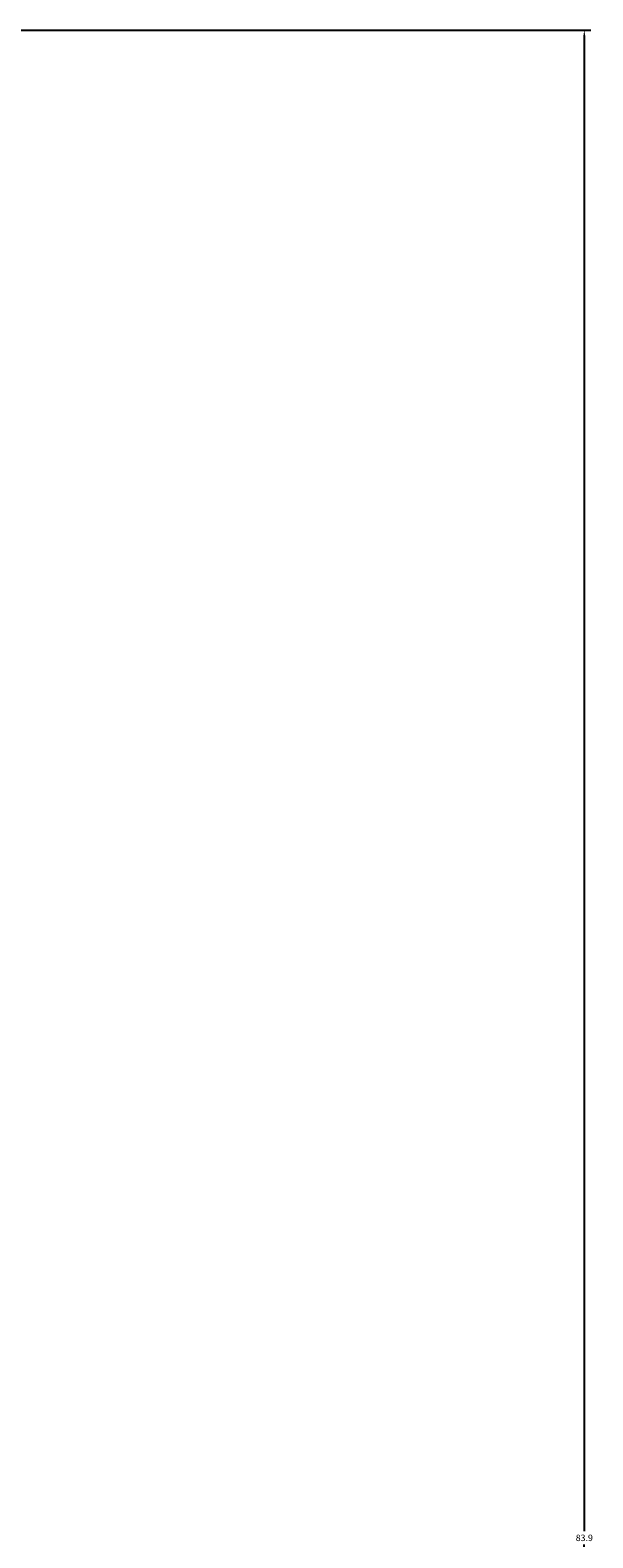
# Model space of a CAD drawing. Units: feet. Extents: x 2695 to 2912, y 795 to 1139.
# Tile 64 of 83: x 2896 to 2911, y 979 to 1021. Entities that reach past the tile are written whole.
import ezdxf

# ---------------------------------------------------------------- set-up
doc = ezdxf.new("R2010")
doc.units = ezdxf.units.FT
doc.layers.add('A-ANNO-DIMS', color=2, linetype='Continuous', lineweight=18)
doc.styles.get("Standard").update_dxf_attribs({"font": 'arial.ttf'})
doc.dimstyles.get("Standard").update_dxf_attribs({"dimtxt": 0.18, "dimasz": 0.18, "dimexe": 0.18, "dimexo": 0.0625, "dimgap": 0.09, "dimtad": 0, "dimtih": 1, "dimtoh": 1, "dimdec": 1, "dimzin": 0, "dimdsep": 46, "dimlunit": 3, "dimtxsty": 'Standard', "dimcen": 0.09, "dimadec": 0, "dimazin": 0, "dimtfac": 1, "dimtdec": 1, "dimtofl": 0, "dimtmove": 0, "dimatfit": 3, "dimfxl": 1, "dimtolj": 1, "dimtzin": 0, "dimarcsym": 0})

# ---------------------------------------------------------------- blocks, each defined once
blk = doc.blocks.new('*D17')
at = {"layer": 'A-ANNO-DIMS', "color": 0, "lineweight": -2, "transparency": 16777216}
for p, q in [((2843.637, 1020.824), (2911.424, 1020.824)), ((2911.244, 1020.644), (2911.244, 979.059)), ((2911.244, 937.111), (2911.244, 978.695)), ((2890.699, 936.931), (2911.424, 936.931))]:
    blk.add_line(p, q, dxfattribs=at)
at = {"layer": 'A-ANNO-DIMS', "color": 0, "transparency": 16777216}
for points in [[(2911.214, 1020.644), (2911.274, 1020.644), (2911.244, 1020.824)], [(2911.214, 937.111), (2911.274, 937.111), (2911.244, 936.931)]]:
    blk.add_solid(points, dxfattribs=at)
at = {"layer": 'Defpoints', "color": 0, "transparency": 16777216}
for p in [(2843.575, 1020.824), (2911.244, 1020.824), (2890.636, 936.931)]:
    blk.add_point(p, dxfattribs=at)
at = {"layer": 'A-ANNO-DIMS', "color": 0, "transparency": 16777216, "insert": (2911.244, 978.877), "char_height": 0.18, "attachment_point": 5}
blk.add_mtext('\\A1;83.9', dxfattribs=at)

msp = doc.modelspace()

# ---------------------------------------------------------------- dimensions: what is measured, and where the dimension line sits
at = {"layer": 'A-ANNO-DIMS'}
dim = msp.add_linear_dim(base=(2911.2444, 1020.8235), p1=(2890.6361, 936.9306), p2=(2843.575, 1020.8235), angle=90, dimstyle='Standard', override={"dimdec": 1, "dimlfac": 1, "dimrnd": 0, "dimzin": 0, "dimdsep": 46, "dimlunit": 2}, dxfattribs=at)
dim.commit()
dim.dimension.update_dxf_attribs({"geometry": '*D17', "text_midpoint": (2911.2444, 978.877)})

doc.saveas('drawing.dxf')
